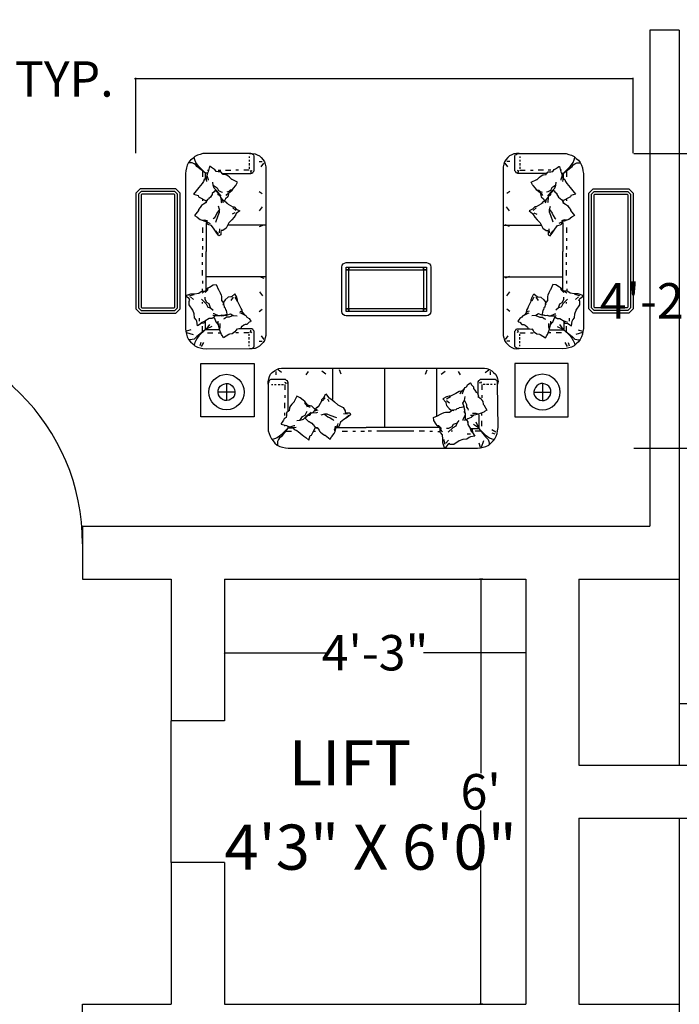
# Model space of a CAD drawing. Units: inches. Extents: x -113 to 5399, y -1393 to 3302.
# Tile 28 of 40: x 3870 to 3982, y 189 to 356. Entities that reach past the tile are written whole.
import ezdxf

# ---------------------------------------------------------------- set-up
doc = ezdxf.new("R2010")
doc.units = ezdxf.units.IN
doc.header["$MEASUREMENT"] = 0
doc.layers.add('24', color=7, linetype='Continuous')
for name, color, linetype, lineweight in [('A-ANNO-DIMS', 254, 'Continuous', 18), ('A-AREA-IDEN', 4, 'Continuous', 18), ('doors', 2, 'Continuous', 25), ('furniture', 131, 'Continuous', 18), ('walls', 1, 'Continuous', 25)]:
    doc.layers.add(name, color=color, linetype=linetype, lineweight=lineweight)
doc.styles.get("Standard").update_dxf_attribs({"font": 'arial.ttf'})
doc.dimstyles.get("Standard").update_dxf_attribs({"dimtxt": 6, "dimasz": 0.18, "dimexe": 0.18, "dimexo": 0.0625, "dimgap": 0.09, "dimtad": 0, "dimtih": 1, "dimtoh": 1, "dimdec": 1, "dimzin": 0, "dimdsep": 46, "dimlunit": 4, "dimtxsty": 'Standard', "dimblk": 'ARCHTICK', "dimcen": 0.09, "dimadec": 0, "dimazin": 0, "dimtfac": 1, "dimtdec": 1, "dimtofl": 0, "dimtmove": 0, "dimatfit": 3, "dimfxl": 1, "dimtolj": 1, "dimtzin": 0, "dimarcsym": 0})

# ---------------------------------------------------------------- blocks, each defined once
blk = doc.blocks.new('*U3')
for p, q in [((0, 0), (0, -6)), ((36, 0), (36, -6))]:
    blk.add_line(p, q)
blk.add_lwpolyline([(0, 0), (0, 36), (1.75, 36), (1.75, 0)], close=True)
blk.add_arc((0, 0), 36, 0, 90)
blk = doc.blocks.new('DL13712')
at = {"layer": '24'}
for p, q in [((33, 28.5), (-34, 28.5)), ((33.5, -29.5), (-10, -29.5))]:
    blk.add_line(p, q, dxfattribs=at)
blk = doc.blocks.new('DL13976')
at = {"layer": '24'}
for p, q in [((-16, 11), (-13.5, 14)), ((-13.5, 14), (-10.5, 16.5)), ((-10.5, 16.5), (-7, 18.5)), ((-7, 18.5), (-3.5, 19.5)), ((-3.5, 19.5), (0.5, 20)), ((0.5, 20), (4.5, 19.5)), ((4.5, 19.5), (8, 18.5)), ((8, 18.5), (11.5, 16.5)), ((11.5, 16.5), (14.5, 14)), ((14.5, 14), (17, 11)), ((-19.5, 0), (-19, 4)), ((-19, -4), (-19.5, 0)), ((-19, 4), (-18, 7.5)), ((-18, 7.5), (-16, 11)), ((-9, 2), (-8, 4.5)), ((-9, -0.5), (-9, 2)), ((-9, 0), (10, 0)), ((-8, 4.5), (-6.5, 6.5)), ((-6.5, 6.5), (-4.5, 8)), ((-5.5, 0), (6.5, 0)), ((-4.5, 8), (-2.5, 9)), ((-2.5, 9), (0, 9.5)), ((0, 9.5), (2.5, 9.5)), ((0.5, -9.5), (0.5, 9.5)), ((0.5, -6), (0.5, 6)), ((2.5, 9.5), (5, 8.5)), ((5, 8.5), (7, 7)), ((7, 7), (8.5, 5)), ((8.5, 5), (9.5, 3)), ((9.5, 3), (10, 0.5)), ((10, 0.5), (10, -2)), ((17, 11), (19, 7.5)), ((19, 7.5), (20, 4)), ((20, 4), (20.5, 0)), ((20.5, 0), (20, -4)), ((-18, -7.5), (-19, -4)), ((-16, -11), (-18, -7.5)), ((-13.5, -14), (-16, -11)), ((-8.5, -3), (-9, -0.5)), ((-7.5, -5), (-8.5, -3)), ((-6, -7), (-7.5, -5)), ((-4, -8.5), (-6, -7)), ((-1.5, -9.5), (-4, -8.5)), ((1, -9.5), (-1.5, -9.5)), ((3.5, -9), (1, -9.5)), ((5.5, -8), (3.5, -9)), ((7.5, -6.5), (5.5, -8)), ((9, -4.5), (7.5, -6.5)), ((10, -2), (9, -4.5)), ((17, -11), (14.5, -14)), ((19, -7.5), (17, -11)), ((20, -4), (19, -7.5)), ((-10.5, -16.5), (-13.5, -14)), ((-7, -18.5), (-10.5, -16.5)), ((-3.5, -19.5), (-7, -18.5)), ((0.5, -20), (-3.5, -19.5)), ((4.5, -19.5), (0.5, -20)), ((8, -18.5), (4.5, -19.5)), ((11.5, -16.5), (8, -18.5)), ((14.5, -14), (11.5, -16.5))]:
    blk.add_line(p, q, dxfattribs=at)
blk = doc.blocks.new('DL13329')
at = {"layer": '24'}
for p, q in [((0, 0), (0, -60)), ((60, 0), (0, 0)), ((60, -60), (60, 0)), ((0, -60), (60, -60))]:
    blk.add_line(p, q, dxfattribs=at)
blk = doc.blocks.new('DL13303')
at = {"layer": '24'}
for p, q in [((-70, 20), (-65, 25)), ((-65, 25), (65, 25)), ((65, 25), (70, 20)), ((-70, -20), (-70, 20)), ((-67, 19), (-64, 22)), ((-67, -19), (-67, 19)), ((-64, 22), (64, 22)), ((-64, 18), (-63, 19)), ((-64, -18), (-64, 18)), ((-63, 19), (63, 19)), ((63, 19), (64, 18)), ((64, 22), (67, 19)), ((64, 18), (64, -18)), ((67, 19), (67, -19)), ((70, 20), (70, -20)), ((-65, -25), (-70, -20)), ((-64, -22), (-67, -19)), ((-63, -19), (-64, -18)), ((64, -22), (-64, -22)), ((63, -19), (-63, -19)), ((64, -18), (63, -19)), ((67, -19), (64, -22)), ((70, -20), (65, -25)), ((65, -25), (-65, -25))]:
    blk.add_line(p, q, dxfattribs=at)
blk = doc.blocks.new('DL12701')
at = {"layer": '24'}
for p, q in [((-96.5, 43.5), (-93.5, 44.5)), ((-93.5, 44.5), (-90, 45)), ((-90, 45), (-87, 45.5)), ((-87, 45.5), (0, 45.5)), ((0, 45.5), (87, 45.5)), ((50, 45), (48, 39.5)), ((51.5, 44.5), (50, 45)), ((53.5, 41.5), (51.5, 44.5)), ((87, 45.5), (90.5, 45)), ((88.5, 39.5), (90, 44.5)), ((90.5, 45), (93.5, 44.5)), ((91.5, 44.5), (94, 37)), ((93.5, 44.5), (96.5, 43.5)), ((-107.5, 32), (-106, 35)), ((-106, 35), (-104, 37.5)), ((-102.5, 35), (-105, 36)), ((-104, 37.5), (-102, 40)), ((-99.5, 34), (-102.5, 35)), ((-102, 40), (-99.5, 42)), ((-99.5, 42), (-96.5, 43.5)), ((-97, 32), (-99.5, 34)), ((-99, 40), (-99, 42)), ((-99, 38), (-99, 40)), ((-98, 36), (-99, 38)), ((-97, 34), (-98, 36)), ((-95, 33), (-97, 34)), ((-69.5, 32), (-67.5, 33.5)), ((-67.5, 33.5), (-64, 36.5)), ((-64, 36.5), (-62.5, 31.5)), ((-45.5, 31), (-40, 35.5)), ((-40, 35.5), (-38.5, 33)), ((48, 35.5), (47.5, 30.5)), ((48, 39.5), (48, 35.5)), ((50.5, 41.5), (49, 36)), ((51.5, 40), (54.5, 36.5)), ((55.5, 40.5), (53.5, 41.5)), ((56, 41.5), (55.5, 40.5)), ((60.5, 41.5), (56, 41.5)), ((66.5, 37.5), (60.5, 41.5)), ((70.5, 36), (66.5, 37.5)), ((75, 35.5), (70.5, 36)), ((77.5, 33.5), (75, 35.5)), ((79, 33), (77.5, 33.5)), ((96, 33), (97.5, 34.5)), ((96.5, 43.5), (99.5, 42)), ((97.5, 34.5), (99, 36)), ((98, 32.5), (100.5, 34)), ((99, 36), (99.5, 38)), ((99.5, 42), (102, 40)), ((100, 40), (99.5, 42)), ((99.5, 38), (100, 40)), ((100.5, 34), (103, 35)), ((102, 40), (104.5, 37.5)), ((103, 35), (106, 36)), ((104.5, 37.5), (106.5, 35)), ((106.5, 35), (108, 32)), ((-109.5, 26), (-108.5, 29)), ((-109.5, 22.5), (-109.5, 26)), ((-109.5, -26.5), (-109.5, 22.5)), ((-108.5, 29), (-107.5, 32)), ((-95, 30.5), (-97, 32)), ((-87.5, 23), (-95, 33)), ((-87.5, 23), (-95, 30.5)), ((-89.5, 26.5), (-83.5, 26.5)), ((-87.5, 21), (-87.5, 23)), ((-81.5, 23), (-87.5, 23)), ((-85, 21.5), (-82, 22.5)), ((-82, 22.5), (-80.5, 24.5)), ((-82, 22.5), (-80.5, 22.5)), ((-80.5, 24.5), (-78, 25.5)), ((-80.5, 24.5), (-80.5, 23.5)), ((-80.5, 22.5), (-78, 22)), ((-78, 25.5), (-76, 27)), ((-77, 25.5), (-77, 25.5)), ((-76, 27), (-71.5, 30.5)), ((-71.5, 30.5), (-69.5, 32)), ((-62.5, 31.5), (-61, 31)), ((-61, 31), (-59.5, 28)), ((-59.5, 28), (-57.5, 24.5)), ((-58, 26.5), (-56.5, 26.5)), ((-58, 21), (-54.5, 23)), ((-57.5, 24.5), (-56.5, 22)), ((-56.5, 22.5), (-54.5, 22.5)), ((-54.5, 22.5), (-52.5, 25.5)), ((-54.5, 23), (-54.5, 22.5)), ((-54, 22.5), (-54, 22.5)), ((-52.5, 25.5), (-52, 26.5)), ((-52, 26.5), (-51, 27.5)), ((-51, 27.5), (-49, 29)), ((-49, 29), (-46.5, 31)), ((-46.5, 31), (-45.5, 31)), ((-38.5, 33), (-38, 32.5)), ((-38, 32.5), (-35.5, 29)), ((-35.5, 29), (-34.5, 27)), ((-34.5, 27), (-35, 24.5)), ((-35, 24.5), (-34.5, 23)), ((-34.5, 27), (-33.5, 24)), ((-34.5, 23), (-34, 21)), ((-33.5, 24), (-33, 22)), ((-32, 22.5), (0.5, 22.5)), ((-26.5, 26.5), (-20.5, 26.5)), ((-14.5, 26.5), (-11.5, 26.5)), ((-5.5, 26.5), (-1.5, 26.5)), ((44, 22.5), (0.5, 22.5)), ((6.5, 26.5), (2.5, 26.5)), ((15.5, 26.5), (12.5, 26.5)), ((27.5, 26.5), (21.5, 26.5)), ((33.5, 26.5), (36.5, 26.5)), ((42.5, 27), (45, 27)), ((45, 23.5), (43.5, 22)), ((45.5, 28), (45, 27)), ((45, 27), (45, 23.5)), ((45, 23.5), (46.5, 26)), ((46.5, 23.5), (45, 22)), ((47.5, 30.5), (45.5, 28)), ((46.5, 26), (47.5, 27)), ((54.5, 23.5), (52, 23.5)), ((54, 27.5), (59.5, 22.5)), ((58, 21.5), (54.5, 23.5)), ((59, 26.5), (57.5, 26.5)), ((59.5, 22.5), (63, 20.5)), ((79, 30), (75.5, 30)), ((76, 19), (79, 24)), ((84, 32), (79, 33)), ((80.5, 28), (79, 24)), ((79, 24), (81, 24.5)), ((79, 23.5), (88.5, 23.5)), ((81, 24.5), (81.5, 28)), ((81.5, 28), (84, 32)), ((82.5, 18.5), (88, 22.5)), ((90.5, 26.5), (84.5, 26.5)), ((85, 16), (88, 22.5)), ((88.5, 23.5), (96, 33)), ((88.5, 23.5), (95.5, 30.5)), ((88.5, 8), (88.5, 23.5)), ((95.5, 30.5), (98, 32.5)), ((103, 28.5), (106.5, 29.5)), ((107.5, 27.5), (103, 25)), ((108, 32), (109, 29)), ((109, 29), (109.5, 26)), ((109.5, 26), (110, 22.5)), ((110, 22.5), (109.5, -26.5)), ((-95, 18.5), (-92, 19.5)), ((-95, 18), (-95, 18.5)), ((-94, 16.5), (-95, 18)), ((-92.5, 14), (-94, 16.5)), ((-92, 13.5), (-92.5, 14)), ((-92, 19.5), (-89, 20)), ((-91.5, 12.5), (-92, 13.5)), ((-89.5, 11), (-91.5, 12.5)), ((-91, 21), (-91, 19.5)), ((-89, 20), (-87.5, 21)), ((-87.5, 21), (-85, 21.5)), ((-85, 21.5), (-80.5, 20)), ((-80.5, 20), (-79.5, 20)), ((-74, 14.5), (-77.5, 15)), ((-70.5, 13.5), (-74, 14.5)), ((-74, 14.5), (-71, 10)), ((-67.5, 10.5), (-70.5, 13.5)), ((-68, 12), (-67.5, 12.5)), ((-65, 9), (-68, 12)), ((-67.5, 12.5), (-66.5, 13.5)), ((-66.5, 13.5), (-64.5, 15.5)), ((-64.5, 15.5), (-63.5, 15.5)), ((-63.5, 15.5), (-62.5, 16.5)), ((-62.5, 16.5), (-60.5, 17.5)), ((-60.5, 17.5), (-59, 19.5)), ((-59, 19.5), (-58.5, 19.5)), ((-58.5, 19.5), (-58, 21)), ((-42.5, 10.5), (-40, 11.5)), ((-40, 11.5), (-37, 13.5)), ((-32.5, 11.5), (-40, 9)), ((-37, 13.5), (-36, 14.5)), ((-30, 21), (-33, 22)), ((-33, 22), (-31.5, 19.5)), ((-31.5, 19.5), (-31, 18)), ((-29.5, 19.5), (-30, 21)), ((-28.5, 16.5), (-29.5, 19.5)), ((-24.5, 13.5), (-28.5, 16.5)), ((-21, 11), (-24.5, 13.5)), ((-19, 8.5), (-22.5, 11.5)), ((38, 14), (37.5, 11)), ((40.5, 18.5), (38, 14.5)), ((38, 14.5), (38, 14)), ((41.5, 20), (40.5, 18.5)), ((43.5, 22), (41.5, 20)), ((43.5, 20.5), (41.5, 20)), ((45, 22), (43.5, 20.5)), ((59.5, 19), (58, 21.5)), ((64, 17.5), (59.5, 19)), ((63, 20.5), (64, 17.5)), ((64, 17.5), (66.5, 14.5)), ((70.5, 13.5), (70.5, 14.5)), ((73, 8.5), (70.5, 13.5)), ((73, 13), (72.5, 15)), ((73, 12.5), (75, 14.5)), ((73, 12.5), (73, 13)), ((73, 8.5), (73, 12.5)), ((76, 12.5), (74, 14)), ((75, 14.5), (76, 16)), ((75.5, 16), (76, 16.5)), ((76, 16), (76, 19)), ((80, 11), (76, 12.5)), ((92, 21), (92, 15)), ((-91, 9), (-91, 6)), ((-91, 0.5), (-91, -5.5)), ((-89, 9), (-89.5, 11)), ((-89, 8.5), (-89, 9)), ((-89, 6), (-89, 8.5)), ((-86.5, 3.5), (-89, 6)), ((-87, 3.5), (-87, -26.5)), ((-86, 3.5), (-86.5, 3.5)), ((-85.5, 0.5), (-86, 3.5)), ((-85.5, 0), (-85.5, 0.5)), ((-84.5, -2), (-85.5, 0)), ((-71, 10), (-68, 8.5)), ((-68, 8.5), (-66.5, 5.5)), ((-61.5, 5.5), (-67.5, 10.5)), ((-66.5, 5.5), (-66, 4)), ((-63, 9), (-65, 9)), ((-62.5, 0), (-63.5, -1)), ((-62, 6.5), (-63, 9)), ((-60, 6), (-62, 6.5)), ((-61, -2), (-58.5, 0.5)), ((-57.5, 3.5), (-60, 6)), ((-60, 6), (-55, 5.5)), ((-58.5, 0.5), (-55.5, 2)), ((-56.5, 3.5), (-57.5, 3.5)), ((-57.5, 3.5), (-56, 1.5)), ((-54, 3), (-56.5, 3.5)), ((-56, 1.5), (-55, 0)), ((-55, 5.5), (-54, 5)), ((-55, 0), (-52.5, -2.5)), ((-46.5, 7.5), (-50.5, 8.5)), ((-46.5, 7.5), (-42.5, 10.5)), ((-43.5, 7.5), (-46.5, 7.5)), ((-40, 9), (-43.5, 7.5)), ((-31.5, -3), (-25.5, 0)), ((-25.5, 0), (-23, 3.5)), ((-20.5, 7.5), (-25, 7)), ((-23, 5.5), (-21.5, 6)), ((-23, 3.5), (-23, 5.5)), ((-21.5, 6), (-18, 6)), ((-17, 8), (-21, 11)), ((-18, 6), (-17, 8)), ((37.5, 11), (43.5, 8.5)), ((43.5, 8.5), (44, 8)), ((44, 8), (47, 6.5)), ((47, 6.5), (49.5, 5.5)), ((49.5, 5.5), (51, 5)), ((51, 5), (52.5, 5)), ((52, -2.5), (55, 1)), ((52.5, 5), (55.5, 5)), ((55, 1), (57.5, 3)), ((55.5, 5), (55.5, 5)), ((55.5, 5), (59, 2.5)), ((59, 2.5), (60, 3.5)), ((60, 3.5), (60, 2.5)), ((60, 2.5), (63, 2)), ((63, 2), (64, 1)), ((64, 1), (66, 0.5)), ((66, 0.5), (66.5, 0)), ((66.5, 0), (69, -0.5)), ((71.5, -1), (72.5, 2.5)), ((72, 5), (73, 6.5)), ((73, 5.5), (72, -1)), ((72.5, 2.5), (72, 5)), ((73, 6.5), (73, 8.5)), ((74.5, -0.5), (76, 1.5)), ((76, 1.5), (76.5, 3)), ((80.5, 9), (79, 9)), ((80.5, 10.5), (80, 11)), ((83, 8.5), (80.5, 10.5)), ((83, 8.5), (80.5, 9)), ((84, 6.5), (81.5, 6.5)), ((85, 8), (83, 8.5)), ((85.5, 6.5), (84, 6.5)), ((88, 7.5), (85, 8)), ((88, 7.5), (85.5, 6.5)), ((90, 6.5), (88, 7.5)), ((94, 5), (90, 6.5)), ((92, 9), (92, 6)), ((95, 4.5), (94, 5)), ((94, -3), (97.5, 3)), ((97.5, 3), (95, 4.5)), ((-91, -14), (-91, -11)), ((-83, -4), (-84.5, -2)), ((-80.5, -6.5), (-83, -4)), ((-80.5, -7), (-80.5, -6.5)), ((-77.5, -13), (-80.5, -7)), ((-73.5, -11), (-74.5, -11.5)), ((-70.5, -8.5), (-73.5, -11)), ((-68.5, -7), (-70.5, -8.5)), ((-68.5, -4.5), (-67, -3)), ((-66.5, -4.5), (-68.5, -7)), ((-68.5, -7), (-68.5, -4.5)), ((-67, -3), (-66, -1)), ((-65.5, -3), (-66.5, -4.5)), ((-63.5, -1), (-65.5, -3)), ((-65.5, -3), (-62.5, -2.5)), ((-62.5, -2.5), (-61, -2)), ((-54, -0.5), (-53.5, -0.5)), ((-52.5, -2.5), (-49.5, -7.5)), ((-49.5, -7.5), (-49.5, -9)), ((-49.5, -9), (-47, -11.5)), ((-45.5, -11), (-48.5, -7.5)), ((-43, -10), (-41.5, -7)), ((-42, -11.5), (-41, -11)), ((-41, -11), (-38, -9)), ((-38, -9), (-35, -6.5)), ((-35, -6.5), (-31.5, -3)), ((48, -10), (51.5, -6)), ((52, -12), (48, -10)), ((51.5, -5.5), (52, -2.5)), ((51.5, -6), (51.5, -5.5)), ((52, -8), (55.5, -5.5)), ((52, -10), (56.5, -12.5)), ((69, -0.5), (70.5, -1)), ((70.5, -1), (71.5, -1)), ((72, -1), (70.5, -5)), ((70.5, -5), (72.5, -8)), ((72.5, -8), (74.5, -3.5)), ((72.5, -8), (73, -12.5)), ((74.5, -3.5), (74.5, -0.5)), ((87.5, -12.5), (89.5, -11)), ((89.5, -11), (91, -10)), ((91, -10), (92, -8.5)), ((92, -8.5), (93, -7)), ((92, -14), (92, -11)), ((93, -7), (93.5, -4)), ((93.5, -4), (94, -3)), ((-91, -26), (-91, -20)), ((-74.5, -11.5), (-77.5, -13)), ((-47, -11.5), (-45, -15.5)), ((-45, -15.5), (-42, -11.5)), ((55, -13), (52, -12)), ((56.5, -13), (55, -13)), ((62.5, -16), (56.5, -13)), ((64.5, -17), (62.5, -16)), ((64, -16.5), (64, -16.5)), ((66.5, -18), (64.5, -17)), ((69, -18.5), (66.5, -18)), ((67.5, -15.5), (68.5, -18)), ((68.5, -18), (69, -18.5)), ((69, -18.5), (72, -21)), ((70, -16.5), (69.5, -15.5)), ((72, -21), (70, -16.5)), ((72, -21), (73, -22.5)), ((82.5, -21.5), (83.5, -20)), ((82.5, -22.5), (82.5, -21.5)), ((83.5, -20), (85, -18)), ((85, -17.5), (87, -16.5)), ((85, -18), (85, -17.5)), ((87, -16.5), (88, -13)), ((88, -13), (87.5, -12.5)), ((87.5, -26.5), (87.5, -14.5)), ((92, -26), (92, -20)), ((-109.5, -28), (-109.5, -26.5)), ((-109.5, -26.5), (-109.5, -29.5)), ((-109, -29), (-109.5, -28)), ((-109.5, -29.5), (-109, -32.5)), ((-108.5, -30), (-109, -29)), ((-109, -32.5), (-108, -35)), ((-108, -31), (-108.5, -30)), ((-106.5, -31.5), (-108, -31)), ((-105.5, -31.5), (-106.5, -31.5)), ((-106, -26), (-104.5, -26)), ((-104.5, -31.5), (-105.5, -31.5)), ((-92, -31.5), (-104.5, -31.5)), ((-102.5, -26), (-100.5, -26)), ((-98.5, -26), (-96, -26)), ((-94.5, -26), (-92.5, -26)), ((-91, -31.5), (-92, -31.5)), ((-90, -31.5), (-91, -31.5)), ((-90.5, -27.5), (-88, -28)), ((-90.5, -28), (-90, -29)), ((-89, -30.5), (-90, -31.5)), ((-88, -30), (-89, -30.5)), ((-87.5, -29), (-88, -30)), ((-87, -28), (-87.5, -29)), ((-87, -26.5), (-87, -28)), ((73, -22.5), (74.5, -23.5)), ((74.5, -23.5), (76, -26)), ((76, -26), (79, -28)), ((79, -28), (79.5, -27.5)), ((79.5, -27.5), (80, -26)), ((80, -26), (82.5, -23.5)), ((82.5, -23.5), (82.5, -22.5)), ((87.5, -28), (87.5, -26.5)), ((87.5, -29), (87.5, -28)), ((88, -30), (87.5, -29)), ((89, -30.5), (88, -30)), ((91.5, -27.5), (89, -28)), ((90, -31.5), (89, -30.5)), ((91, -31.5), (90, -31.5)), ((91.5, -28), (91, -29)), ((92.5, -31.5), (91, -31.5)), ((104.5, -31.5), (92.5, -31.5)), ((95.5, -26), (93.5, -26)), ((99.5, -26), (97, -26)), ((103.5, -26), (101.5, -26)), ((106, -31.5), (104.5, -31.5)), ((107, -26), (105.5, -26)), ((107, -31.5), (106, -31.5)), ((108, -31), (107, -31.5)), ((109, -30), (108, -31)), ((108.5, -35), (109.5, -32.5)), ((109.5, -29), (109, -30)), ((110, -29.5), (109.5, -26.5)), ((109.5, -26.5), (109.5, -28)), ((109.5, -28), (109.5, -29)), ((109.5, -32.5), (110, -29.5)), ((-108, -35), (-107, -37.5)), ((-107, -37.5), (-105, -39.5)), ((-105, -39.5), (-102.5, -41.5)), ((-102.5, -41.5), (-100, -43)), ((-100.5, -37), (-100.5, -40.5)), ((-100, -43), (-97.5, -44)), ((-94.5, -39.5), (-98.5, -42.5)), ((-97.5, -44), (-94.5, -44.5)), ((-67, -37), (-64.5, -40.5)), ((-45, -37.5), (-49.5, -41)), ((-27.5, -37.5), (-29.5, -42.5)), ((28.5, -37.5), (30.5, -42.5)), ((46, -37.5), (50.5, -41)), ((68, -37), (65.5, -40.5)), ((95, -44.5), (97.5, -44)), ((95.5, -39.5), (99.5, -42.5)), ((97.5, -44), (100.5, -43)), ((100.5, -43), (103, -41.5)), ((101.5, -37), (101.5, -40.5)), ((103, -41.5), (105, -39.5)), ((105, -39.5), (107, -37.5)), ((107, -37.5), (108.5, -35)), ((-94.5, -44.5), (0, -44.5)), ((0, -44.5), (95, -44.5))]:
    blk.add_line(p, q, dxfattribs=at)
blk = doc.blocks.new('DL13707')
at = {"layer": '24'}
for p, q in [((0, -33.5), (0, 33.5)), ((-58.5, -33.5), (-58.5, 21.5)), ((58.5, -33.5), (58.5, 2))]:
    blk.add_line(p, q, dxfattribs=at)
blk = doc.blocks.new('DL13651')
at = {"layer": '24'}
for p, q in [((-50.5, 25), (-50, 27)), ((-50.5, -25), (-50.5, 25)), ((-50, 27), (-49, 28.5)), ((-49, 28.5), (-47.5, 29.5)), ((-47.5, 29.5), (-45.5, 30)), ((-45.5, 30), (44.5, 30)), ((-45.5, 24.5), (-45.5, 25)), ((-45.5, 25), (-45, 25)), ((-45.5, -24.5), (-45.5, 24.5)), ((-45, 25), (44, 25)), ((-42.5, -24.5), (-42.5, 24.5)), ((-42.5, 24.5), (-42.5, 22)), ((41.5, 22), (41.5, 24.5)), ((41.5, 24.5), (41.5, -24.5)), ((44, 25), (44.5, 25)), ((44.5, 30), (46.5, 29.5)), ((44.5, 25), (44.5, 24.5)), ((44.5, 24.5), (44.5, -24.5)), ((46.5, 29.5), (48, 28.5)), ((48, 28.5), (49, 27)), ((49, 27), (49.5, 25)), ((49.5, 25), (49.5, -25)), ((-45, 22), (44, 22)), ((-42.5, 22), (-45, 22)), ((44, 22), (41.5, 22)), ((44, -22), (-45, -22)), ((-45, -22), (-42.5, -22)), ((-42.5, -22), (-42.5, -24.5)), ((41.5, -24.5), (41.5, -22)), ((41.5, -22), (44, -22)), ((-50, -27), (-50.5, -25)), ((-49, -28.5), (-50, -27)), ((-47.5, -29.5), (-49, -28.5)), ((-45.5, -30), (-47.5, -29.5)), ((-45.5, -25), (-45.5, -24.5)), ((-45, -25), (-45.5, -25)), ((44.5, -30), (-45.5, -30)), ((44, -25), (-45, -25)), ((44.5, -25), (44, -25)), ((44.5, -24.5), (44.5, -25)), ((46.5, -29.5), (44.5, -30)), ((48, -28.5), (46.5, -29.5)), ((49, -27), (48, -28.5)), ((49.5, -25), (49, -27))]:
    blk.add_line(p, q, dxfattribs=at)
blk = doc.blocks.new('DL12263')
at = {"layer": '24'}
for p, q in [((-115.5, 43.5), (-112.5, 44.5)), ((-112.5, 44.5), (-109, 45)), ((-109, 45), (-106, 45.5)), ((-106, 45.5), (-19, 45.5)), ((-19, 45.5), (106.5, 45.5)), ((69.5, 45), (67.5, 39.5)), ((71, 44.5), (69.5, 45)), ((73, 41.5), (71, 44.5)), ((106.5, 45.5), (110, 45)), ((108, 39.5), (109.5, 44.5)), ((110, 45), (113, 44.5)), ((111, 44.5), (113.5, 37)), ((113, 44.5), (116, 43.5)), ((-126.5, 32), (-125, 35)), ((-125, 35), (-123, 37.5)), ((-121.5, 35), (-124, 36)), ((-123, 37.5), (-121, 40)), ((-118.5, 34), (-121.5, 35)), ((-121, 40), (-118.5, 42)), ((-118.5, 42), (-115.5, 43.5)), ((-116, 32), (-118.5, 34)), ((-118, 40), (-118, 42)), ((-118, 38), (-118, 40)), ((-117, 36), (-118, 38)), ((-116, 34), (-117, 36)), ((-114, 33), (-116, 34)), ((-88.5, 32), (-86.5, 33.5)), ((-86.5, 33.5), (-83, 36.5)), ((-83, 36.5), (-81.5, 31.5)), ((-64.5, 31), (-59, 35.5)), ((-59, 35.5), (-57.5, 33)), ((67.5, 35.5), (67, 30.5)), ((67.5, 39.5), (67.5, 35.5)), ((70, 41.5), (68.5, 36)), ((71, 40), (74, 36.5)), ((75, 40.5), (73, 41.5)), ((75.5, 41.5), (75, 40.5)), ((80, 41.5), (75.5, 41.5)), ((86, 37.5), (80, 41.5)), ((90, 36), (86, 37.5)), ((94.5, 35.5), (90, 36)), ((97, 33.5), (94.5, 35.5)), ((98.5, 33), (97, 33.5)), ((115.5, 33), (117, 34.5)), ((116, 43.5), (119, 42)), ((117, 34.5), (118.5, 36)), ((117.5, 32.5), (120, 34)), ((118.5, 36), (119, 38)), ((119, 42), (121.5, 40)), ((119.5, 40), (119, 42)), ((119, 38), (119.5, 40)), ((120, 34), (122.5, 35)), ((121.5, 40), (124, 37.5)), ((122.5, 35), (125.5, 36)), ((124, 37.5), (126, 35)), ((126, 35), (127.5, 32)), ((-128.5, 26), (-127.5, 29)), ((-128.5, 22.5), (-128.5, 26)), ((-128.5, -26.5), (-128.5, 22.5)), ((-127.5, 29), (-126.5, 32)), ((-114, 30.5), (-116, 32)), ((-106.5, 23), (-114, 33)), ((-106.5, 23), (-114, 30.5)), ((-108.5, 26.5), (-102.5, 26.5)), ((-106.5, 21), (-106.5, 23)), ((-100.5, 23), (-106.5, 23)), ((-104, 21.5), (-101, 22.5)), ((-101, 22.5), (-99.5, 24.5)), ((-101, 22.5), (-99.5, 22.5)), ((-99.5, 24.5), (-97, 25.5)), ((-99.5, 24.5), (-99.5, 23.5)), ((-99.5, 22.5), (-97, 22)), ((-97, 25.5), (-95, 27)), ((-96, 25.5), (-96, 25.5)), ((-95, 27), (-90.5, 30.5)), ((-90.5, 30.5), (-88.5, 32)), ((-81.5, 31.5), (-80, 31)), ((-80, 31), (-78.5, 28)), ((-78.5, 28), (-76.5, 24.5)), ((-77, 26.5), (-75.5, 26.5)), ((-77, 21), (-73.5, 23)), ((-76.5, 24.5), (-75.5, 22)), ((-75.5, 22.5), (-73.5, 22.5)), ((-73.5, 22.5), (-71.5, 25.5)), ((-73.5, 23), (-73.5, 22.5)), ((-73, 22.5), (-73, 22.5)), ((-71.5, 25.5), (-71, 26.5)), ((-71, 26.5), (-70, 27.5)), ((-70, 27.5), (-68, 29)), ((-68, 29), (-65.5, 31)), ((-65.5, 31), (-64.5, 31)), ((-57.5, 33), (-57, 32.5)), ((-57, 32.5), (-54.5, 29)), ((-54.5, 29), (-53.5, 27)), ((-53.5, 27), (-54, 24.5)), ((-54, 24.5), (-53.5, 23)), ((-53.5, 27), (-52.5, 24)), ((-53.5, 23), (-53, 21)), ((-52.5, 24), (-52, 22)), ((-51, 22.5), (-18.5, 22.5)), ((-45.5, 26.5), (-39.5, 26.5)), ((-33.5, 26.5), (-30.5, 26.5)), ((-24.5, 26.5), (-20.5, 26.5)), ((63.5, 22.5), (-18.5, 22.5)), ((-12.5, 26.5), (-16.5, 26.5)), ((35, 26.5), (-6.5, 26.5)), ((47, 26.5), (41, 26.5)), ((53, 26.5), (56, 26.5)), ((62, 27), (64.5, 27)), ((64.5, 23.5), (63, 22)), ((65, 28), (64.5, 27)), ((64.5, 27), (64.5, 23.5)), ((64.5, 23.5), (66, 26)), ((66, 23.5), (64.5, 22)), ((67, 30.5), (65, 28)), ((66, 26), (67, 27)), ((74, 23.5), (71.5, 23.5)), ((73.5, 27.5), (79, 22.5)), ((77.5, 21.5), (74, 23.5)), ((78.5, 26.5), (77, 26.5)), ((79, 22.5), (82.5, 20.5)), ((98.5, 30), (95, 30)), ((95.5, 19), (98.5, 24)), ((103.5, 32), (98.5, 33)), ((100, 28), (98.5, 24)), ((98.5, 24), (100.5, 24.5)), ((98.5, 23.5), (108, 23.5)), ((100.5, 24.5), (101, 28)), ((101, 28), (103.5, 32)), ((102, 18.5), (107.5, 22.5)), ((110, 26.5), (104, 26.5)), ((104.5, 16), (107.5, 22.5)), ((108, 23.5), (115.5, 33)), ((108, 23.5), (115, 30.5)), ((108, 8), (108, 23.5)), ((115, 30.5), (117.5, 32.5)), ((122.5, 28.5), (126, 29.5)), ((127, 27.5), (122.5, 25)), ((127.5, 32), (128.5, 29)), ((128.5, 29), (129, 26)), ((129, 26), (129.5, 22.5)), ((129.5, 22.5), (129, -26.5)), ((-114, 18.5), (-111, 19.5)), ((-114, 18), (-114, 18.5)), ((-113, 16.5), (-114, 18)), ((-111.5, 14), (-113, 16.5)), ((-111, 13.5), (-111.5, 14)), ((-111, 19.5), (-108, 20)), ((-110.5, 12.5), (-111, 13.5)), ((-108.5, 11), (-110.5, 12.5)), ((-110, 21), (-110, 19.5)), ((-108, 20), (-106.5, 21)), ((-106.5, 21), (-104, 21.5)), ((-104, 21.5), (-99.5, 20)), ((-99.5, 20), (-98.5, 20)), ((-93, 14.5), (-96.5, 15)), ((-89.5, 13.5), (-93, 14.5)), ((-93, 14.5), (-90, 10)), ((-86.5, 10.5), (-89.5, 13.5)), ((-87, 12), (-86.5, 12.5)), ((-84, 9), (-87, 12)), ((-86.5, 12.5), (-85.5, 13.5)), ((-85.5, 13.5), (-83.5, 15.5)), ((-83.5, 15.5), (-82.5, 15.5)), ((-82.5, 15.5), (-81.5, 16.5)), ((-81.5, 16.5), (-79.5, 17.5)), ((-79.5, 17.5), (-78, 19.5)), ((-78, 19.5), (-77.5, 19.5)), ((-77.5, 19.5), (-77, 21)), ((-61.5, 10.5), (-59, 11.5)), ((-59, 11.5), (-56, 13.5)), ((-51.5, 11.5), (-59, 9)), ((-56, 13.5), (-55, 14.5)), ((-49, 21), (-52, 22)), ((-52, 22), (-50.5, 19.5)), ((-50.5, 19.5), (-50, 18)), ((-48.5, 19.5), (-49, 21)), ((-47.5, 16.5), (-48.5, 19.5)), ((-43.5, 13.5), (-47.5, 16.5)), ((-40, 11), (-43.5, 13.5)), ((-38, 8.5), (-41.5, 11.5)), ((57.5, 14), (57, 11)), ((60, 18.5), (57.5, 14.5)), ((57.5, 14.5), (57.5, 14)), ((61, 20), (60, 18.5)), ((63, 22), (61, 20)), ((63, 20.5), (61, 20)), ((64.5, 22), (63, 20.5)), ((79, 19), (77.5, 21.5)), ((83.5, 17.5), (79, 19)), ((82.5, 20.5), (83.5, 17.5)), ((83.5, 17.5), (86, 14.5)), ((90, 13.5), (90, 14.5)), ((92.5, 8.5), (90, 13.5)), ((92.5, 13), (92, 15)), ((92.5, 12.5), (94.5, 14.5)), ((92.5, 12.5), (92.5, 13)), ((92.5, 8.5), (92.5, 12.5)), ((95.5, 12.5), (93.5, 14)), ((94.5, 14.5), (95.5, 16)), ((95, 16), (95.5, 16.5)), ((95.5, 16), (95.5, 19)), ((99.5, 11), (95.5, 12.5)), ((111.5, 21), (111.5, 15)), ((-110, 9), (-110, 6)), ((-110, 0.5), (-110, -5.5)), ((-108, 9), (-108.5, 11)), ((-108, 8.5), (-108, 9)), ((-108, 6), (-108, 8.5)), ((-105.5, 3.5), (-108, 6)), ((-106, 3.5), (-106, -26.5)), ((-105, 3.5), (-105.5, 3.5)), ((-104.5, 0.5), (-105, 3.5)), ((-104.5, 0), (-104.5, 0.5)), ((-103.5, -2), (-104.5, 0)), ((-90, 10), (-87, 8.5)), ((-87, 8.5), (-85.5, 5.5)), ((-80.5, 5.5), (-86.5, 10.5)), ((-85.5, 5.5), (-85, 4)), ((-82, 9), (-84, 9)), ((-81.5, 0), (-82.5, -1)), ((-81, 6.5), (-82, 9)), ((-79, 6), (-81, 6.5)), ((-80, -2), (-77.5, 0.5)), ((-76.5, 3.5), (-79, 6)), ((-79, 6), (-74, 5.5)), ((-77.5, 0.5), (-74.5, 2)), ((-75.5, 3.5), (-76.5, 3.5)), ((-76.5, 3.5), (-75, 1.5)), ((-73, 3), (-75.5, 3.5)), ((-75, 1.5), (-74, 0)), ((-74, 5.5), (-73, 5)), ((-74, 0), (-71.5, -2.5)), ((-65.5, 7.5), (-69.5, 8.5)), ((-65.5, 7.5), (-61.5, 10.5)), ((-62.5, 7.5), (-65.5, 7.5)), ((-59, 9), (-62.5, 7.5)), ((-50.5, -3), (-44.5, 0)), ((-44.5, 0), (-42, 3.5)), ((-39.5, 7.5), (-44, 7)), ((-42, 5.5), (-40.5, 6)), ((-42, 3.5), (-42, 5.5)), ((-40.5, 6), (-37, 6)), ((-36, 8), (-40, 11)), ((-37, 6), (-36, 8)), ((57, 11), (63, 8.5)), ((63, 8.5), (63.5, 8)), ((63.5, 8), (66.5, 6.5)), ((66.5, 6.5), (69, 5.5)), ((69, 5.5), (70.5, 5)), ((70.5, 5), (72, 5)), ((71.5, -2.5), (74.5, 1)), ((72, 5), (75, 5)), ((74.5, 1), (77, 3)), ((75, 5), (75, 5)), ((75, 5), (78.5, 2.5)), ((78.5, 2.5), (79.5, 3.5)), ((79.5, 3.5), (79.5, 2.5)), ((79.5, 2.5), (82.5, 2)), ((82.5, 2), (83.5, 1)), ((83.5, 1), (85.5, 0.5)), ((85.5, 0.5), (86, 0)), ((86, 0), (88.5, -0.5)), ((91, -1), (92, 2.5)), ((91.5, 5), (92.5, 6.5)), ((92.5, 5.5), (91.5, -1)), ((92, 2.5), (91.5, 5)), ((92.5, 6.5), (92.5, 8.5)), ((94, -0.5), (95.5, 1.5)), ((95.5, 1.5), (96, 3)), ((100, 9), (98.5, 9)), ((100, 10.5), (99.5, 11)), ((102.5, 8.5), (100, 10.5)), ((102.5, 8.5), (100, 9)), ((103.5, 6.5), (101, 6.5)), ((104.5, 8), (102.5, 8.5)), ((105, 6.5), (103.5, 6.5)), ((107.5, 7.5), (104.5, 8)), ((107.5, 7.5), (105, 6.5)), ((109.5, 6.5), (107.5, 7.5)), ((113.5, 5), (109.5, 6.5)), ((111.5, 9), (111.5, 6)), ((114.5, 4.5), (113.5, 5)), ((113.5, -3), (117, 3)), ((117, 3), (114.5, 4.5)), ((-110, -14), (-110, -11)), ((-102, -4), (-103.5, -2)), ((-99.5, -6.5), (-102, -4)), ((-99.5, -7), (-99.5, -6.5)), ((-96.5, -13), (-99.5, -7)), ((-92.5, -11), (-93.5, -11.5)), ((-89.5, -8.5), (-92.5, -11)), ((-87.5, -7), (-89.5, -8.5)), ((-87.5, -4.5), (-86, -3)), ((-85.5, -4.5), (-87.5, -7)), ((-87.5, -7), (-87.5, -4.5)), ((-86, -3), (-85, -1)), ((-84.5, -3), (-85.5, -4.5)), ((-82.5, -1), (-84.5, -3)), ((-84.5, -3), (-81.5, -2.5)), ((-81.5, -2.5), (-80, -2)), ((-73, -0.5), (-72.5, -0.5)), ((-71.5, -2.5), (-68.5, -7.5)), ((-68.5, -7.5), (-68.5, -9)), ((-68.5, -9), (-66, -11.5)), ((-64.5, -11), (-67.5, -7.5)), ((-62, -10), (-60.5, -7)), ((-61, -11.5), (-60, -11)), ((-60, -11), (-57, -9)), ((-57, -9), (-54, -6.5)), ((-54, -6.5), (-50.5, -3)), ((67.5, -10), (71, -6)), ((71.5, -12), (67.5, -10)), ((71, -5.5), (71.5, -2.5)), ((71, -6), (71, -5.5)), ((71.5, -8), (75, -5.5)), ((71.5, -10), (76, -12.5)), ((88.5, -0.5), (90, -1)), ((90, -1), (91, -1)), ((91.5, -1), (90, -5)), ((90, -5), (92, -8)), ((92, -8), (94, -3.5)), ((92, -8), (92.5, -12.5)), ((94, -3.5), (94, -0.5)), ((107, -12.5), (109, -11)), ((109, -11), (110.5, -10)), ((110.5, -10), (111.5, -8.5)), ((111.5, -8.5), (112.5, -7)), ((111.5, -14), (111.5, -11)), ((112.5, -7), (113, -4)), ((113, -4), (113.5, -3)), ((-110, -26), (-110, -20)), ((-93.5, -11.5), (-96.5, -13)), ((-66, -11.5), (-64, -15.5)), ((-64, -15.5), (-61, -11.5)), ((74.5, -13), (71.5, -12)), ((76, -13), (74.5, -13)), ((82, -16), (76, -13)), ((84, -17), (82, -16)), ((83.5, -16.5), (83.5, -16.5)), ((86, -18), (84, -17)), ((88.5, -18.5), (86, -18)), ((87, -15.5), (88, -18)), ((88, -18), (88.5, -18.5)), ((88.5, -18.5), (91.5, -21)), ((89.5, -16.5), (89, -15.5)), ((91.5, -21), (89.5, -16.5)), ((91.5, -21), (92.5, -22.5)), ((102, -21.5), (103, -20)), ((102, -22.5), (102, -21.5)), ((103, -20), (104.5, -18)), ((104.5, -17.5), (106.5, -16.5)), ((104.5, -18), (104.5, -17.5)), ((106.5, -16.5), (107.5, -13)), ((107.5, -13), (107, -12.5)), ((107, -26.5), (107, -14.5)), ((111.5, -26), (111.5, -20)), ((-128.5, -28), (-128.5, -26.5)), ((-128.5, -26.5), (-128.5, -29.5)), ((-128, -29), (-128.5, -28)), ((-128.5, -29.5), (-128, -32.5)), ((-127.5, -30), (-128, -29)), ((-128, -32.5), (-127, -35)), ((-127, -31), (-127.5, -30)), ((-125.5, -31.5), (-127, -31)), ((-124.5, -31.5), (-125.5, -31.5)), ((-125, -26), (-123.5, -26)), ((-123.5, -31.5), (-124.5, -31.5)), ((-111, -31.5), (-123.5, -31.5)), ((-121.5, -26), (-119.5, -26)), ((-117.5, -26), (-115, -26)), ((-113.5, -26), (-111.5, -26)), ((-110, -31.5), (-111, -31.5)), ((-109, -31.5), (-110, -31.5)), ((-109.5, -27.5), (-107, -28)), ((-109.5, -28), (-109, -29)), ((-108, -30.5), (-109, -31.5)), ((-107, -30), (-108, -30.5)), ((-106.5, -29), (-107, -30)), ((-106, -28), (-106.5, -29)), ((-106, -26.5), (-106, -28)), ((92.5, -22.5), (94, -23.5)), ((94, -23.5), (95.5, -26)), ((95.5, -26), (98.5, -28)), ((98.5, -28), (99, -27.5)), ((99, -27.5), (99.5, -26)), ((99.5, -26), (102, -23.5)), ((102, -23.5), (102, -22.5)), ((107, -28), (107, -26.5)), ((107, -29), (107, -28)), ((107.5, -30), (107, -29)), ((108.5, -30.5), (107.5, -30)), ((111, -27.5), (108.5, -28)), ((109.5, -31.5), (108.5, -30.5)), ((110.5, -31.5), (109.5, -31.5)), ((111, -28), (110.5, -29)), ((112, -31.5), (110.5, -31.5)), ((124, -31.5), (112, -31.5)), ((115, -26), (113, -26)), ((119, -26), (116.5, -26)), ((123, -26), (121, -26)), ((125.5, -31.5), (124, -31.5)), ((126.5, -26), (125, -26)), ((126.5, -31.5), (125.5, -31.5)), ((127.5, -31), (126.5, -31.5)), ((128.5, -30), (127.5, -31)), ((128, -35), (129, -32.5)), ((129, -29), (128.5, -30)), ((129.5, -29.5), (129, -26.5)), ((129, -26.5), (129, -28)), ((129, -28), (129, -29)), ((129, -32.5), (129.5, -29.5)), ((-127, -35), (-126, -37.5)), ((-126, -37.5), (-124, -39.5)), ((-124, -39.5), (-121.5, -41.5)), ((-121.5, -41.5), (-119, -43)), ((-119.5, -37), (-119.5, -40.5)), ((-119, -43), (-116.5, -44)), ((-113.5, -39.5), (-117.5, -42.5)), ((-116.5, -44), (-113.5, -44.5)), ((-86, -37), (-83.5, -40.5)), ((-64, -37.5), (-68.5, -41)), ((-46.5, -37.5), (-48.5, -42.5)), ((48, -37.5), (50, -42.5)), ((65.5, -37.5), (70, -41)), ((87.5, -37), (85, -40.5)), ((114.5, -44.5), (117, -44)), ((115, -39.5), (119, -42.5)), ((117, -44), (120, -43)), ((120, -43), (122.5, -41.5)), ((121, -37), (121, -40.5)), ((122.5, -41.5), (124.5, -39.5)), ((124.5, -39.5), (126.5, -37.5)), ((126.5, -37.5), (128, -35)), ((-113.5, -44.5), (-19, -44.5)), ((-19, -44.5), (114.5, -44.5))]:
    blk.add_line(p, q, dxfattribs=at)
blk = doc.blocks.new('U3M')
at = {"yscale": 10, "zscale": 10}
for name, p, xscale, rotation in [('DL13303', (1315, 2544), -10, 180), ('DL13712', (1310, 1664), -10, 90), ('DL13976', (-270, 1769), 10, 90), ('DL12263', (-445, 20), -10, 90), ('DL13707', (-335, 0), 10, 90), ('DL13651', (885, -25), 10, 270), ('DL12701', (1315, -1779), 10, 180), ('DL13712', (1310, -1664), 10, 90), ('DL13329', (50, -2064), 10, 180), ('DL13976', (-270, -1769), -10, 90)]:
    blk.add_blockref(name, p, dxfattribs=dict(at, xscale=xscale, rotation=rotation))
for name, p, xscale in [('DL12701', (1315, 1779), -10), ('DL13329', (50, 2064), -10), ('DL13303', (1315, -2544), 10)]:
    blk.add_blockref(name, p, dxfattribs=dict(at, xscale=xscale))
at = {"flags": 3}
for tag in ['AECLAY', 'AECGTYPE']:
    blk.add_attdef(tag, (0, 0), '', height=0.5, dxfattribs=at)
blk = doc.blocks.new('_ArchTick')
at = {"color": 0, "linetype": 'ByBlock', "const_width": 0.15}
blk.add_lwpolyline([(-0.5, -0.5), (0.5, 0.5)], dxfattribs=at)
blk = doc.blocks.new('*D95')
at = {"layer": 'A-ANNO-DIMS', "color": 0, "lineweight": -2, "transparency": 16777216}
for p, q in [((3948.45, 260.78), (3947.93, 260.78)), ((3948.11, 260.78), (3948.11, 227.93)), ((3948.11, 188.78), (3948.11, 221.62)), ((3948.45, 188.78), (3947.93, 188.78))]:
    blk.add_line(p, q, dxfattribs=at)
at = {"layer": 'Defpoints', "color": 0, "transparency": 16777216}
for p in [(3948.51, 260.78), (3948.11, 188.78), (3948.51, 188.78)]:
    blk.add_point(p, dxfattribs=at)
at = {"layer": 'A-ANNO-DIMS', "color": 0, "lineweight": -2, "transparency": 16777216, "xscale": 0.18, "yscale": 0.18, "zscale": 0.18}
for p, rotation in [((3948.11, 260.78), 90), ((3948.11, 188.78), 270)]:
    blk.add_blockref('_ArchTick', p, dxfattribs=dict(at, rotation=rotation))
at = {"layer": 'A-ANNO-DIMS', "color": 0, "transparency": 16777216, "insert": (3948.11, 224.78), "char_height": 6, "attachment_point": 5}
blk.add_mtext("\\A1;6'", dxfattribs=at)
blk = doc.blocks.new('*D96')
at = {"layer": 'A-ANNO-DIMS', "color": 0, "lineweight": -2, "transparency": 16777216}
for p, q in [((3904.73, 248.71), (3904.73, 248.14)), ((3955.73, 248.71), (3955.73, 248.14)), ((3904.73, 248.32), (3922.04, 248.32)), ((3955.73, 248.32), (3938.41, 248.32))]:
    blk.add_line(p, q, dxfattribs=at)
at = {"layer": 'Defpoints', "color": 0, "transparency": 16777216}
for p in [(3904.73, 248.78), (3955.73, 248.78), (3955.73, 248.32)]:
    blk.add_point(p, dxfattribs=at)
at = {"layer": 'A-ANNO-DIMS', "color": 0, "lineweight": -2, "transparency": 16777216, "xscale": 0.18, "yscale": 0.18, "zscale": 0.18, "rotation": 180}
blk.add_blockref('_ArchTick', (3904.73, 248.32), dxfattribs=at)
at = {"layer": 'A-ANNO-DIMS', "color": 0, "lineweight": -2, "transparency": 16777216, "xscale": 0.18, "yscale": 0.18, "zscale": 0.18}
blk.add_blockref('_ArchTick', (3955.73, 248.32), dxfattribs=at)
at = {"layer": 'A-ANNO-DIMS', "color": 0, "transparency": 16777216, "insert": (3930.23, 248.32), "char_height": 6, "attachment_point": 5}
blk.add_mtext('\\A1;4\'-3"', dxfattribs=at)
blk = doc.blocks.new('*D122')
at = {"layer": 'A-ANNO-DIMS', "color": 0, "lineweight": -2, "transparency": 16777216}
for p, q in [((3981.73, 243.83), (3981.73, 239.54)), ((4113.73, 243.83), (4113.73, 239.54)), ((3981.73, 239.72), (4042.83, 239.72)), ((4113.73, 239.72), (4052.63, 239.72))]:
    blk.add_line(p, q, dxfattribs=at)
at = {"layer": 'Defpoints', "color": 0, "transparency": 16777216}
for p in [(3981.73, 243.89), (4113.73, 243.89), (4113.73, 239.72)]:
    blk.add_point(p, dxfattribs=at)
at = {"layer": 'A-ANNO-DIMS', "color": 0, "lineweight": -2, "transparency": 16777216, "xscale": 0.18, "yscale": 0.18, "zscale": 0.18, "rotation": 180}
blk.add_blockref('_ArchTick', (3981.73, 239.72), dxfattribs=at)
at = {"layer": 'A-ANNO-DIMS', "color": 0, "lineweight": -2, "transparency": 16777216, "xscale": 0.18, "yscale": 0.18, "zscale": 0.18}
blk.add_blockref('_ArchTick', (4113.73, 239.72), dxfattribs=at)
at = {"layer": 'A-ANNO-DIMS', "color": 0, "transparency": 16777216, "insert": (4047.73, 239.72), "char_height": 6, "attachment_point": 5}
blk.add_mtext("\\A1;11'", dxfattribs=at)
blk = doc.blocks.new('*D185')
at = {"layer": 'A-ANNO-DIMS', "color": 0, "lineweight": -2, "transparency": 16777216}
for p, q in [((3889.72, 345.5), (3889.54, 345.5)), ((3889.72, 332.93), (3889.72, 345.68)), ((3973.94, 345.5), (3889.72, 345.5)), ((3973.94, 332.93), (3973.94, 345.68))]:
    blk.add_line(p, q, dxfattribs=at)
at = {"layer": 'Defpoints', "color": 0, "transparency": 16777216}
for p in [(3889.72, 345.5), (3889.72, 332.87), (3973.94, 332.87)]:
    blk.add_point(p, dxfattribs=at)
at = {"layer": 'A-ANNO-DIMS', "color": 0, "lineweight": -2, "transparency": 16777216, "xscale": 0.18, "yscale": 0.18, "zscale": 0.18, "rotation": 180}
blk.add_blockref('_ArchTick', (3889.72, 345.5), dxfattribs=at)
at = {"layer": 'A-ANNO-DIMS', "color": 0, "lineweight": -2, "transparency": 16777216, "xscale": 0.18, "yscale": 0.18, "zscale": 0.18}
blk.add_blockref('_ArchTick', (3973.94, 345.5), dxfattribs=at)
at = {"layer": 'A-ANNO-DIMS', "color": 0, "transparency": 16777216, "insert": (3835.08, 345.5), "char_height": 6, "attachment_point": 5}
blk.add_mtext('\\A1;SEATING GROUP 7\'-0" TYP.', dxfattribs=at)
blk = doc.blocks.new('*D186')
at = {"layer": 'A-ANNO-DIMS', "color": 0, "lineweight": -2, "transparency": 16777216}
for p, q in [((3974.01, 332.87), (3986.76, 332.87)), ((3986.58, 332.87), (3986.58, 311.03)), ((3986.58, 282.98), (3986.58, 304.82)), ((3974.01, 282.98), (3986.76, 282.98))]:
    blk.add_line(p, q, dxfattribs=at)
at = {"layer": 'Defpoints', "color": 0, "transparency": 16777216}
for p in [(3973.94, 332.87), (3986.58, 332.87), (3973.94, 282.98)]:
    blk.add_point(p, dxfattribs=at)
at = {"layer": 'A-ANNO-DIMS', "color": 0, "lineweight": -2, "transparency": 16777216, "xscale": 0.18, "yscale": 0.18, "zscale": 0.18}
for p, rotation in [((3986.58, 332.87), 90), ((3986.58, 282.98), 270)]:
    blk.add_blockref('_ArchTick', p, dxfattribs=dict(at, rotation=rotation))
at = {"layer": 'A-ANNO-DIMS', "color": 0, "transparency": 16777216, "insert": (3986.58, 307.92), "char_height": 6, "attachment_point": 5}
blk.add_mtext('\\A1;4\'-2" TYP.', dxfattribs=at)
blk = doc.blocks.new('*D210')
at = {"layer": 'A-ANNO-DIMS', "color": 0, "lineweight": -2, "transparency": 16777216}
for p, q in [((3839.79, 561.28), (4159.21, 561.28)), ((4159.03, 561.28), (4159.03, 230.43)), ((4159.03, -106.72), (4159.03, 224.12)), ((3839.79, -106.72), (4159.21, -106.72))]:
    blk.add_line(p, q, dxfattribs=at)
at = {"layer": 'Defpoints', "color": 0, "transparency": 16777216}
for p in [(3839.73, 561.28), (4159.03, 561.28), (3839.73, -106.72)]:
    blk.add_point(p, dxfattribs=at)
at = {"layer": 'A-ANNO-DIMS', "color": 0, "lineweight": -2, "transparency": 16777216, "xscale": 0.18, "yscale": 0.18, "zscale": 0.18}
for p, rotation in [((4159.03, 561.28), 90), ((4159.03, -106.72), 270)]:
    blk.add_blockref('_ArchTick', p, dxfattribs=dict(at, rotation=rotation))
at = {"layer": 'A-ANNO-DIMS', "color": 0, "transparency": 16777216, "insert": (4159.03, 227.28), "char_height": 6, "attachment_point": 5}
blk.add_mtext('\\A1;55\'-8"', dxfattribs=at)

msp = doc.modelspace()

# ---------------------------------------------------------------- linework, layer by layer
at = {"layer": 'walls'}
for p, q in [((3976.73, 353.78), (3976.73, 269.78)), ((3981.73, 353.78), (3976.73, 353.78)), ((3981.73, 353.78), (3981.73, 229.28)), ((3880.73, 269.78), (3976.73, 269.78)), ((3880.73, 269.78), (3880.73, 260.78)), ((3880.73, 260.78), (3895.73, 260.78)), ((3895.73, 260.78), (3895.73, 236.78)), ((3904.73, 260.78), (3904.73, 236.78)), ((3904.73, 260.78), (3955.73, 260.78)), ((3955.73, 260.78), (3955.73, 188.78)), ((3964.73, 260.78), (3964.73, 229.28)), ((3964.73, 260.78), (3981.73, 260.78)), ((3904.73, 236.78), (3895.73, 236.78)), ((3895.73, 212.78), (3895.73, 236.78)), ((3964.73, 229.28), (4113.73, 229.28)), ((3964.73, 220.28), (3964.73, 188.78)), ((3964.73, 220.28), (4113.73, 220.28)), ((3981.73, 220.28), (3981.73, 88.28)), ((3895.73, 212.78), (3895.73, 188.78)), ((3904.73, 212.78), (3895.73, 212.78)), ((3904.73, 212.78), (3904.73, 188.78)), ((3880.73, 188.78), (3895.73, 188.78)), ((3904.73, 188.78), (3955.73, 188.78)), ((3964.73, 188.78), (3981.73, 188.78))]:
    msp.add_line(p, q, dxfattribs=at)

# ---------------------------------------------------------------- block references
at = {"layer": 'doors'}
msp.add_blockref('*U3', (3844.73, 266.78), dxfattribs=at)
at = {"layer": 'doors', "xscale": -1, "rotation": 180}
msp.add_blockref('*U3', (3844.73, 182.78), dxfattribs=at)
at = {"layer": 'furniture', "xscale": 0.0150724250692195, "yscale": 0.0150724250692195, "zscale": 0.0150724250692195, "rotation": 90}
msp.add_blockref('U3M', (3931.83, 296.54), dxfattribs=at)

# ---------------------------------------------------------------- texts
at = {"layer": 'A-AREA-IDEN'}
for s, height, p in [('LIFT', 7.647, (3915.62, 225.84)), ('4\'3" X 6\'0"', 7.6473, (3904.73, 211.57))]:
    msp.add_text(s, height=height, dxfattribs=at).set_placement(p)

# ---------------------------------------------------------------- dimensions: what is measured, and where the dimension line sits
at = {"layer": 'A-ANNO-DIMS'}
for base, p1, p2, override, picture, middle in [((4159.03, 561.28), (3839.73, -106.72), (3839.73, 561.28), {"dimdec": 1, "dimlfac": 1, "dimrnd": 0, "dimzin": 1, "dimdsep": 46, "dimlunit": 4, "dimfrac": 2}, '*D210', (4159.03, 227.28)), ((3948.11, 188.78), (3948.51, 260.78), (3948.51, 188.78), {"dimclrd": 0, "dimclre": 0, "dimclrt": 0}, '*D95', (3948.11, 224.78))]:
    dim = msp.add_linear_dim(base=base, p1=p1, p2=p2, angle=90, dimstyle='Standard', override=override, dxfattribs=at)
    dim.commit()
    dim.dimension.update_dxf_attribs({"geometry": picture, "text_midpoint": middle})
for base, p1, p2, angle, text, picture, middle in [((3889.72, 345.5), (3973.94, 332.87), (3889.72, 332.87), 180, 'SEATING GROUP <> TYP.', '*D185', (3835.08, 345.5)), ((3986.58, 332.87), (3973.94, 282.98), (3973.94, 332.87), 90, '<> TYP.', '*D186', (3986.58, 307.92))]:
    dim = msp.add_linear_dim(base=base, p1=p1, p2=p2, angle=angle, text=text, dimstyle='Standard', override={"dimdec": 1, "dimlfac": 1, "dimrnd": 0, "dimzin": 1, "dimdsep": 46, "dimlunit": 4, "dimfrac": 2}, dxfattribs=at)
    dim.commit()
    dim.dimension.update_dxf_attribs({"geometry": picture, "text_midpoint": middle})
for base, p1, p2, picture, middle in [((3955.73, 248.32), (3904.73, 248.78), (3955.73, 248.78), '*D96', (3930.23, 248.32)), ((4113.73, 239.72), (3981.73, 243.89), (4113.73, 243.89), '*D122', (4047.73, 239.72))]:
    dim = msp.add_linear_dim(base=base, p1=p1, p2=p2, dimstyle='Standard', override={"dimclrd": 0, "dimclre": 0, "dimclrt": 0}, dxfattribs=at)
    dim.commit()
    dim.dimension.update_dxf_attribs({"geometry": picture, "text_midpoint": middle})

doc.saveas('drawing.dxf')
